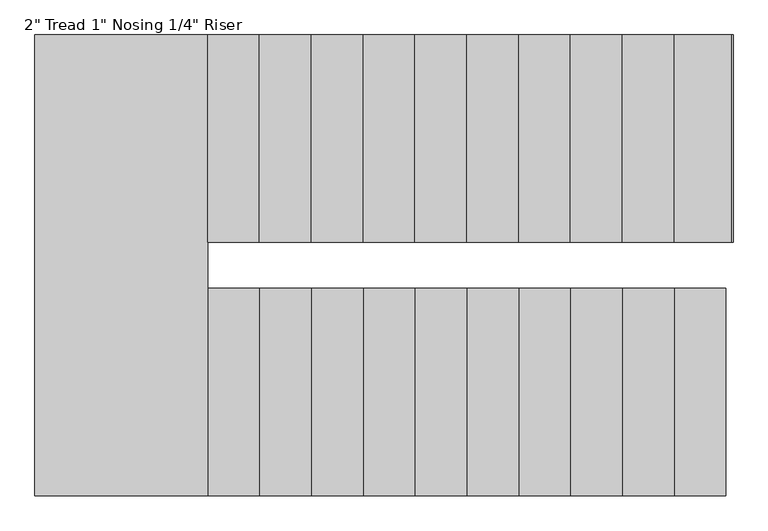
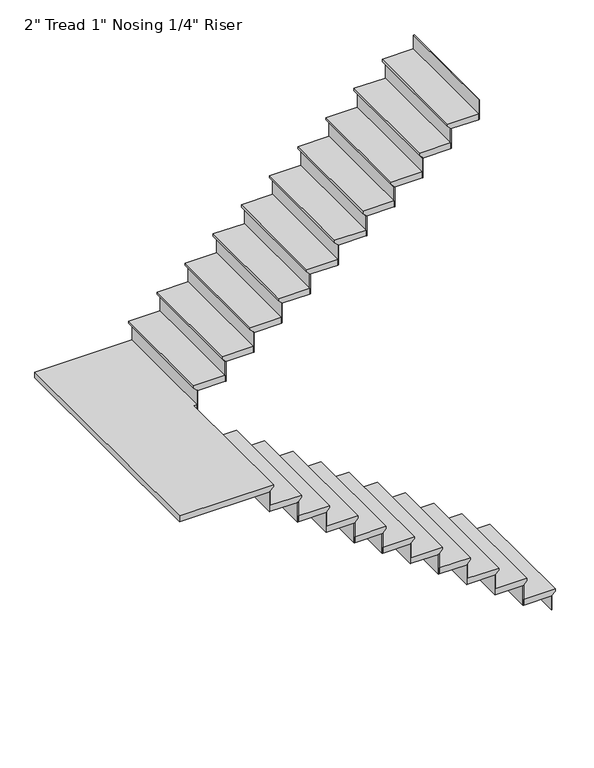
"""IFC4 building model written with IfcOpenShell, lengths in millimetres: stair flight geometry."""

from ifc_helpers import new_model, si_unit, origin, place, context, project, spatial, faceted_brep, source, transform, mapped, element, save


def stair_flight_66f938e6(model_context):
    return source(origin(), model_context, "Body", "Brep", [
        faceted_brep([(-2080.8410855, 332.1803617, 150.2833333), (-2080.8410855, 332.1803617, 169.3333333), (-2080.8410855, -582.2196383, 169.3333333), (-2080.8410855, -582.2196383, 150.2833333), (-2106.2410855, 332.1803617, 124.8833333), (-2106.2410855, -582.2196383, 124.8833333), (-2334.8410855, 332.1803617, 169.3333333), (-2334.8410855, -582.2196383, 169.3333333), (-2106.2410855, -582.2196383, 118.5333333), (-2334.8410855, -582.2196383, 118.5333333), (-2334.8410855, 332.1803617, 118.5333333), (-2106.2410855, 332.1803617, 118.5333333)], [[[0, 1, 2, 3]], [[4, 0, 3, 5]], [[2, 1, 6, 7]], [[8, 9, 10, 11]], [[2, 7, 9, 8, 5, 3]], [[8, 11, 4, 5]], [[6, 1, 0, 4, 11, 10]], [[7, 6, 10, 9]]]),
        faceted_brep([(-2106.2410855, 332.1803617, 118.5333333), (-2106.2410855, 332.1803617, 0.0), (-2112.5910855, 332.1803617, 0.0), (-2112.5910855, 332.1803617, 118.5333333), (-2106.2410855, -582.2196383, 118.5333333), (-2112.5910855, -582.2196383, 118.5333333), (-2112.5910855, -582.2196383, 0.0), (-2106.2410855, -582.2196383, 0.0)], [[[0, 1, 2, 3]], [[4, 5, 6, 7]], [[1, 0, 4, 7]], [[2, 1, 7, 6]], [[3, 2, 6, 5]], [[0, 3, 5, 4]]]),
        faceted_brep([(-2334.8410855, 332.1803617, 287.8666667), (-2334.8410855, 332.1803617, 118.5333333), (-2341.1910855, 332.1803617, 118.5333333), (-2341.1910855, 332.1803617, 287.8666667), (-2334.8410855, -582.2196383, 287.8666667), (-2341.1910855, -582.2196383, 287.8666667), (-2341.1910855, -582.2196383, 118.5333333), (-2334.8410855, -582.2196383, 118.5333333)], [[[0, 1, 2, 3]], [[4, 5, 6, 7]], [[1, 0, 4, 7]], [[2, 1, 7, 6]], [[3, 2, 6, 5]], [[0, 3, 5, 4]]]),
        faceted_brep([(-2309.4410855, -582.2196383, 338.6666667), (-2309.4410855, 332.1803617, 338.6666667), (-2563.4410855, 332.1803617, 338.6666667), (-2563.4410855, -582.2196383, 338.6666667), (-2334.8410855, -582.2196383, 287.8666667), (-2563.4410855, -582.2196383, 287.8666667), (-2563.4410855, 332.1803617, 287.8666667), (-2334.8410855, 332.1803617, 287.8666667), (-2334.8410855, -582.2196383, 294.2166667), (-2309.4410855, -582.2196383, 319.6166667), (-2334.8410855, 332.1803617, 294.2166667), (-2309.4410855, 332.1803617, 319.6166667)], [[[0, 1, 2, 3]], [[4, 5, 6, 7]], [[0, 3, 5, 4, 8, 9]], [[4, 7, 10, 8]], [[2, 1, 11, 10, 7, 6]], [[3, 2, 6, 5]], [[11, 1, 0, 9]], [[10, 11, 9, 8]]]),
        faceted_brep([(-2563.4410855, 332.1803617, 457.2), (-2563.4410855, 332.1803617, 287.8666667), (-2569.7910855, 332.1803617, 287.8666667), (-2569.7910855, 332.1803617, 457.2), (-2563.4410855, -582.2196383, 457.2), (-2569.7910855, -582.2196383, 457.2), (-2569.7910855, -582.2196383, 287.8666667), (-2563.4410855, -582.2196383, 287.8666667)], [[[0, 1, 2, 3]], [[4, 5, 6, 7]], [[1, 0, 4, 7]], [[2, 1, 7, 6]], [[3, 2, 6, 5]], [[0, 3, 5, 4]]]),
        faceted_brep([(-2538.0410855, -582.2196383, 508.0), (-2538.0410855, 332.1803617, 508.0), (-2792.0410855, 332.1803617, 508.0), (-2792.0410855, -582.2196383, 508.0), (-2563.4410855, -582.2196383, 457.2), (-2792.0410855, -582.2196383, 457.2), (-2792.0410855, 332.1803617, 457.2), (-2563.4410855, 332.1803617, 457.2), (-2563.4410855, -582.2196383, 463.55), (-2538.0410855, -582.2196383, 488.95), (-2563.4410855, 332.1803617, 463.55), (-2538.0410855, 332.1803617, 488.95)], [[[0, 1, 2, 3]], [[4, 5, 6, 7]], [[0, 3, 5, 4, 8, 9]], [[4, 7, 10, 8]], [[2, 1, 11, 10, 7, 6]], [[3, 2, 6, 5]], [[11, 1, 0, 9]], [[10, 11, 9, 8]]]),
        faceted_brep([(-2792.0410855, 332.1803617, 626.5333333), (-2792.0410855, 332.1803617, 457.2), (-2798.3910855, 332.1803617, 457.2), (-2798.3910855, 332.1803617, 626.5333333), (-2792.0410855, -582.2196383, 626.5333333), (-2798.3910855, -582.2196383, 626.5333333), (-2798.3910855, -582.2196383, 457.2), (-2792.0410855, -582.2196383, 457.2)], [[[0, 1, 2, 3]], [[4, 5, 6, 7]], [[1, 0, 4, 7]], [[2, 1, 7, 6]], [[3, 2, 6, 5]], [[0, 3, 5, 4]]]),
        faceted_brep([(-2766.6410855, -582.2196383, 677.3333333), (-2766.6410855, 332.1803617, 677.3333333), (-3020.6410855, 332.1803617, 677.3333333), (-3020.6410855, -582.2196383, 677.3333333), (-2792.0410855, -582.2196383, 626.5333333), (-3020.6410855, -582.2196383, 626.5333333), (-3020.6410855, 332.1803617, 626.5333333), (-2792.0410855, 332.1803617, 626.5333333), (-2792.0410855, -582.2196383, 632.8833333), (-2766.6410855, -582.2196383, 658.2833333), (-2792.0410855, 332.1803617, 632.8833333), (-2766.6410855, 332.1803617, 658.2833333)], [[[0, 1, 2, 3]], [[4, 5, 6, 7]], [[0, 3, 5, 4, 8, 9]], [[4, 7, 10, 8]], [[2, 1, 11, 10, 7, 6]], [[3, 2, 6, 5]], [[11, 1, 0, 9]], [[10, 11, 9, 8]]]),
        faceted_brep([(-3020.6410855, 332.1803617, 795.8666667), (-3020.6410855, 332.1803617, 626.5333333), (-3026.9910855, 332.1803617, 626.5333333), (-3026.9910855, 332.1803617, 795.8666667), (-3020.6410855, -582.2196383, 795.8666667), (-3026.9910855, -582.2196383, 795.8666667), (-3026.9910855, -582.2196383, 626.5333333), (-3020.6410855, -582.2196383, 626.5333333)], [[[0, 1, 2, 3]], [[4, 5, 6, 7]], [[1, 0, 4, 7]], [[2, 1, 7, 6]], [[3, 2, 6, 5]], [[0, 3, 5, 4]]]),
        faceted_brep([(-2995.2410855, -582.2196383, 846.6666667), (-2995.2410855, 332.1803617, 846.6666667), (-3249.2410855, 332.1803617, 846.6666667), (-3249.2410855, -582.2196383, 846.6666667), (-3020.6410855, -582.2196383, 795.8666667), (-3249.2410855, -582.2196383, 795.8666667), (-3249.2410855, 332.1803617, 795.8666667), (-3020.6410855, 332.1803617, 795.8666667), (-3020.6410855, -582.2196383, 802.2166667), (-2995.2410855, -582.2196383, 827.6166667), (-3020.6410855, 332.1803617, 802.2166667), (-2995.2410855, 332.1803617, 827.6166667)], [[[0, 1, 2, 3]], [[4, 5, 6, 7]], [[0, 3, 5, 4, 8, 9]], [[4, 7, 10, 8]], [[2, 1, 11, 10, 7, 6]], [[3, 2, 6, 5]], [[11, 1, 0, 9]], [[10, 11, 9, 8]]]),
        faceted_brep([(-3249.2410855, 332.1803617, 965.2), (-3249.2410855, 332.1803617, 795.8666667), (-3255.5910855, 332.1803617, 795.8666667), (-3255.5910855, 332.1803617, 965.2), (-3249.2410855, -582.2196383, 965.2), (-3255.5910855, -582.2196383, 965.2), (-3255.5910855, -582.2196383, 795.8666667), (-3249.2410855, -582.2196383, 795.8666667)], [[[0, 1, 2, 3]], [[4, 5, 6, 7]], [[1, 0, 4, 7]], [[2, 1, 7, 6]], [[3, 2, 6, 5]], [[0, 3, 5, 4]]]),
        faceted_brep([(-3223.8410855, -582.2196383, 1016.0), (-3223.8410855, 332.1803617, 1016.0), (-3477.8410855, 332.1803617, 1016.0), (-3477.8410855, -582.2196383, 1016.0), (-3249.2410855, -582.2196383, 965.2), (-3477.8410855, -582.2196383, 965.2), (-3477.8410855, 332.1803617, 965.2), (-3249.2410855, 332.1803617, 965.2), (-3249.2410855, -582.2196383, 971.55), (-3223.8410855, -582.2196383, 996.95), (-3249.2410855, 332.1803617, 971.55), (-3223.8410855, 332.1803617, 996.95)], [[[0, 1, 2, 3]], [[4, 5, 6, 7]], [[0, 3, 5, 4, 8, 9]], [[4, 7, 10, 8]], [[2, 1, 11, 10, 7, 6]], [[3, 2, 6, 5]], [[11, 1, 0, 9]], [[10, 11, 9, 8]]]),
        faceted_brep([(-3477.8410855, 332.1803617, 1134.5333333), (-3477.8410855, 332.1803617, 965.2), (-3484.1910855, 332.1803617, 965.2), (-3484.1910855, 332.1803617, 1134.5333333), (-3477.8410855, -582.2196383, 1134.5333333), (-3484.1910855, -582.2196383, 1134.5333333), (-3484.1910855, -582.2196383, 965.2), (-3477.8410855, -582.2196383, 965.2)], [[[0, 1, 2, 3]], [[4, 5, 6, 7]], [[1, 0, 4, 7]], [[2, 1, 7, 6]], [[3, 2, 6, 5]], [[0, 3, 5, 4]]]),
        faceted_brep([(-3452.4410855, -582.2196383, 1185.3333333), (-3452.4410855, 332.1803617, 1185.3333333), (-3706.4410855, 332.1803617, 1185.3333333), (-3706.4410855, -582.2196383, 1185.3333333), (-3477.8410855, -582.2196383, 1134.5333333), (-3706.4410855, -582.2196383, 1134.5333333), (-3706.4410855, 332.1803617, 1134.5333333), (-3477.8410855, 332.1803617, 1134.5333333), (-3477.8410855, -582.2196383, 1140.8833333), (-3452.4410855, -582.2196383, 1166.2833333), (-3477.8410855, 332.1803617, 1140.8833333), (-3452.4410855, 332.1803617, 1166.2833333)], [[[0, 1, 2, 3]], [[4, 5, 6, 7]], [[0, 3, 5, 4, 8, 9]], [[4, 7, 10, 8]], [[2, 1, 11, 10, 7, 6]], [[3, 2, 6, 5]], [[11, 1, 0, 9]], [[10, 11, 9, 8]]]),
        faceted_brep([(-3706.4410855, 332.1803617, 1303.8666667), (-3706.4410855, 332.1803617, 1134.5333333), (-3712.7910855, 332.1803617, 1134.5333333), (-3712.7910855, 332.1803617, 1303.8666667), (-3706.4410855, -582.2196383, 1303.8666667), (-3712.7910855, -582.2196383, 1303.8666667), (-3712.7910855, -582.2196383, 1134.5333333), (-3706.4410855, -582.2196383, 1134.5333333)], [[[0, 1, 2, 3]], [[4, 5, 6, 7]], [[1, 0, 4, 7]], [[2, 1, 7, 6]], [[3, 2, 6, 5]], [[0, 3, 5, 4]]]),
        faceted_brep([(-3681.0410855, -582.2196383, 1354.6666667), (-3681.0410855, 332.1803617, 1354.6666667), (-3935.0410855, 332.1803617, 1354.6666667), (-3935.0410855, -582.2196383, 1354.6666667), (-3706.4410855, -582.2196383, 1303.8666667), (-3935.0410855, -582.2196383, 1303.8666667), (-3935.0410855, 332.1803617, 1303.8666667), (-3706.4410855, 332.1803617, 1303.8666667), (-3706.4410855, -582.2196383, 1310.2166667), (-3681.0410855, -582.2196383, 1335.6166667), (-3706.4410855, 332.1803617, 1310.2166667), (-3681.0410855, 332.1803617, 1335.6166667)], [[[0, 1, 2, 3]], [[4, 5, 6, 7]], [[0, 3, 5, 4, 8, 9]], [[4, 7, 10, 8]], [[2, 1, 11, 10, 7, 6]], [[3, 2, 6, 5]], [[11, 1, 0, 9]], [[10, 11, 9, 8]]]),
        faceted_brep([(-3935.0410855, 332.1803617, 1473.2), (-3935.0410855, 332.1803617, 1303.8666667), (-3941.3910855, 332.1803617, 1303.8666667), (-3941.3910855, 332.1803617, 1473.2), (-3935.0410855, -582.2196383, 1473.2), (-3941.3910855, -582.2196383, 1473.2), (-3941.3910855, -582.2196383, 1303.8666667), (-3935.0410855, -582.2196383, 1303.8666667)], [[[0, 1, 2, 3]], [[4, 5, 6, 7]], [[1, 0, 4, 7]], [[2, 1, 7, 6]], [[3, 2, 6, 5]], [[0, 3, 5, 4]]]),
        faceted_brep([(-3909.6410855, -582.2196383, 1524.0), (-3909.6410855, 332.1803617, 1524.0), (-4163.6410855, 332.1803617, 1524.0), (-4163.6410855, -582.2196383, 1524.0), (-3935.0410855, -582.2196383, 1473.2), (-4163.6410855, -582.2196383, 1473.2), (-4163.6410855, 332.1803617, 1473.2), (-3935.0410855, 332.1803617, 1473.2), (-3935.0410855, -582.2196383, 1479.55), (-3909.6410855, -582.2196383, 1504.95), (-3935.0410855, 332.1803617, 1479.55), (-3909.6410855, 332.1803617, 1504.95)], [[[0, 1, 2, 3]], [[4, 5, 6, 7]], [[0, 3, 5, 4, 8, 9]], [[4, 7, 10, 8]], [[2, 1, 11, 10, 7, 6]], [[3, 2, 6, 5]], [[11, 1, 0, 9]], [[10, 11, 9, 8]]]),
        faceted_brep([(-4163.6410855, 332.1803617, 1642.5333333), (-4163.6410855, 332.1803617, 1473.2), (-4169.9910855, 332.1803617, 1473.2), (-4169.9910855, 332.1803617, 1642.5333333), (-4163.6410855, -582.2196383, 1642.5333333), (-4169.9910855, -582.2196383, 1642.5333333), (-4169.9910855, -582.2196383, 1473.2), (-4163.6410855, -582.2196383, 1473.2)], [[[0, 1, 2, 3]], [[4, 5, 6, 7]], [[1, 0, 4, 7]], [[2, 1, 7, 6]], [[3, 2, 6, 5]], [[0, 3, 5, 4]]]),
        faceted_brep([(-4138.2410855, -582.2196383, 1693.3333333), (-4138.2410855, 332.1803617, 1693.3333333), (-4392.2410855, 332.1803617, 1693.3333333), (-4392.2410855, -582.2196383, 1693.3333333), (-4163.6410855, -582.2196383, 1642.5333333), (-4392.2410855, -582.2196383, 1642.5333333), (-4392.2410855, 332.1803617, 1642.5333333), (-4163.6410855, 332.1803617, 1642.5333333), (-4163.6410855, -582.2196383, 1648.8833333), (-4138.2410855, -582.2196383, 1674.2833333), (-4163.6410855, 332.1803617, 1648.8833333), (-4138.2410855, 332.1803617, 1674.2833333)], [[[0, 1, 2, 3]], [[4, 5, 6, 7]], [[0, 3, 5, 4, 8, 9]], [[4, 7, 10, 8]], [[2, 1, 11, 10, 7, 6]], [[3, 2, 6, 5]], [[11, 1, 0, 9]], [[10, 11, 9, 8]]]),
        faceted_brep([(-4392.2410855, 332.1803617, 1811.8666667), (-4392.2410855, 332.1803617, 1642.5333333), (-4398.5910855, 332.1803617, 1642.5333333), (-4398.5910855, 332.1803617, 1811.8666667), (-4392.2410855, -582.2196383, 1811.8666667), (-4398.5910855, -582.2196383, 1811.8666667), (-4398.5910855, -582.2196383, 1642.5333333), (-4392.2410855, -582.2196383, 1642.5333333)], [[[0, 1, 2, 3]], [[4, 5, 6, 7]], [[1, 0, 4, 7]], [[2, 1, 7, 6]], [[3, 2, 6, 5]], [[0, 3, 5, 4]]]),
        faceted_brep([(-4341.4410855, 1449.7803617, 1862.6666667), (-5128.8410855, 1449.7803617, 1862.6666667), (-5128.8410855, -582.2196383, 1862.6666667), (-4366.8410855, -582.2196383, 1862.6666667), (-4366.8410855, 535.3803617, 1862.6666667), (-4341.4410855, 535.3803617, 1862.6666667), (-5128.8410855, 1449.7803617, 1811.8666667), (-4341.4410855, 1449.7803617, 1811.8666667), (-4341.4410855, 535.3803617, 1811.8666667), (-4366.8410855, 535.3803617, 1811.8666667), (-4366.8410855, 332.1803617, 1811.8666667), (-4392.2410855, 332.1803617, 1811.8666667), (-4392.2410855, -582.2196383, 1811.8666667), (-5128.8410855, -582.2196383, 1811.8666667), (-4392.2410855, -582.2196383, 1818.2166667), (-4366.8410855, -582.2196383, 1843.6166667), (-4392.2410855, 332.1803617, 1818.2166667), (-4366.8410855, 332.1803617, 1843.6166667)], [[[0, 1, 2, 3, 4, 5]], [[6, 7, 8, 9, 10, 11, 12, 13]], [[1, 0, 7, 6]], [[2, 1, 6, 13]], [[3, 2, 13, 12, 14, 15]], [[12, 11, 16, 14]], [[11, 10, 17, 16]], [[4, 3, 15, 17, 10, 9]], [[5, 4, 9, 8]], [[0, 5, 8, 7]], [[15, 14, 16, 17]]]),
        faceted_brep([(-4341.4410855, 535.3803617, 1981.2), (-4341.4410855, 535.3803617, 1811.8666667), (-4335.0910855, 535.3803617, 1811.8666667), (-4335.0910855, 535.3803617, 1981.2), (-4341.4410855, 1449.7803617, 1981.2), (-4335.0910855, 1449.7803617, 1981.2), (-4335.0910855, 1449.7803617, 1811.8666667), (-4341.4410855, 1449.7803617, 1811.8666667)], [[[0, 1, 2, 3]], [[4, 5, 6, 7]], [[1, 0, 4, 7]], [[2, 1, 7, 6]], [[3, 2, 6, 5]], [[0, 3, 5, 4]]]),
        faceted_brep([(-4366.8410855, 1449.7803617, 2032.0), (-4366.8410855, 535.3803617, 2032.0), (-4112.8410855, 535.3803617, 2032.0), (-4112.8410855, 1449.7803617, 2032.0), (-4341.4410855, 1449.7803617, 1981.2), (-4112.8410855, 1449.7803617, 1981.2), (-4112.8410855, 535.3803617, 1981.2), (-4341.4410855, 535.3803617, 1981.2), (-4341.4410855, 1449.7803617, 1987.55), (-4366.8410855, 1449.7803617, 2012.95), (-4341.4410855, 535.3803617, 1987.55), (-4366.8410855, 535.3803617, 2012.95)], [[[0, 1, 2, 3]], [[4, 5, 6, 7]], [[0, 3, 5, 4, 8, 9]], [[4, 7, 10, 8]], [[2, 1, 11, 10, 7, 6]], [[3, 2, 6, 5]], [[11, 1, 0, 9]], [[10, 11, 9, 8]]]),
        faceted_brep([(-4112.8410855, 535.3803617, 2150.5333333), (-4112.8410855, 535.3803617, 1981.2), (-4106.4910855, 535.3803617, 1981.2), (-4106.4910855, 535.3803617, 2150.5333333), (-4112.8410855, 1449.7803617, 2150.5333333), (-4106.4910855, 1449.7803617, 2150.5333333), (-4106.4910855, 1449.7803617, 1981.2), (-4112.8410855, 1449.7803617, 1981.2)], [[[0, 1, 2, 3]], [[4, 5, 6, 7]], [[1, 0, 4, 7]], [[2, 1, 7, 6]], [[3, 2, 6, 5]], [[0, 3, 5, 4]]]),
        faceted_brep([(-4138.2410855, 1449.7803617, 2201.3333333), (-4138.2410855, 535.3803617, 2201.3333333), (-3884.2410855, 535.3803617, 2201.3333333), (-3884.2410855, 1449.7803617, 2201.3333333), (-4112.8410855, 1449.7803617, 2150.5333333), (-3884.2410855, 1449.7803617, 2150.5333333), (-3884.2410855, 535.3803617, 2150.5333333), (-4112.8410855, 535.3803617, 2150.5333333), (-4112.8410855, 1449.7803617, 2156.8833333), (-4138.2410855, 1449.7803617, 2182.2833333), (-4112.8410855, 535.3803617, 2156.8833333), (-4138.2410855, 535.3803617, 2182.2833333)], [[[0, 1, 2, 3]], [[4, 5, 6, 7]], [[0, 3, 5, 4, 8, 9]], [[4, 7, 10, 8]], [[2, 1, 11, 10, 7, 6]], [[3, 2, 6, 5]], [[11, 1, 0, 9]], [[10, 11, 9, 8]]]),
        faceted_brep([(-3884.2410855, 535.3803617, 2319.8666667), (-3884.2410855, 535.3803617, 2150.5333333), (-3877.8910855, 535.3803617, 2150.5333333), (-3877.8910855, 535.3803617, 2319.8666667), (-3884.2410855, 1449.7803617, 2319.8666667), (-3877.8910855, 1449.7803617, 2319.8666667), (-3877.8910855, 1449.7803617, 2150.5333333), (-3884.2410855, 1449.7803617, 2150.5333333)], [[[0, 1, 2, 3]], [[4, 5, 6, 7]], [[1, 0, 4, 7]], [[2, 1, 7, 6]], [[3, 2, 6, 5]], [[0, 3, 5, 4]]]),
        faceted_brep([(-3909.6410855, 1449.7803617, 2370.6666667), (-3909.6410855, 535.3803617, 2370.6666667), (-3655.6410855, 535.3803617, 2370.6666667), (-3655.6410855, 1449.7803617, 2370.6666667), (-3884.2410855, 1449.7803617, 2319.8666667), (-3655.6410855, 1449.7803617, 2319.8666667), (-3655.6410855, 535.3803617, 2319.8666667), (-3884.2410855, 535.3803617, 2319.8666667), (-3884.2410855, 1449.7803617, 2326.2166667), (-3909.6410855, 1449.7803617, 2351.6166667), (-3884.2410855, 535.3803617, 2326.2166667), (-3909.6410855, 535.3803617, 2351.6166667)], [[[0, 1, 2, 3]], [[4, 5, 6, 7]], [[0, 3, 5, 4, 8, 9]], [[4, 7, 10, 8]], [[2, 1, 11, 10, 7, 6]], [[3, 2, 6, 5]], [[11, 1, 0, 9]], [[10, 11, 9, 8]]]),
        faceted_brep([(-3655.6410855, 535.3803617, 2489.2), (-3655.6410855, 535.3803617, 2319.8666667), (-3649.2910855, 535.3803617, 2319.8666667), (-3649.2910855, 535.3803617, 2489.2), (-3655.6410855, 1449.7803617, 2489.2), (-3649.2910855, 1449.7803617, 2489.2), (-3649.2910855, 1449.7803617, 2319.8666667), (-3655.6410855, 1449.7803617, 2319.8666667)], [[[0, 1, 2, 3]], [[4, 5, 6, 7]], [[1, 0, 4, 7]], [[2, 1, 7, 6]], [[3, 2, 6, 5]], [[0, 3, 5, 4]]]),
        faceted_brep([(-3681.0410855, 1449.7803617, 2540.0), (-3681.0410855, 535.3803617, 2540.0), (-3427.0410855, 535.3803617, 2540.0), (-3427.0410855, 1449.7803617, 2540.0), (-3655.6410855, 1449.7803617, 2489.2), (-3427.0410855, 1449.7803617, 2489.2), (-3427.0410855, 535.3803617, 2489.2), (-3655.6410855, 535.3803617, 2489.2), (-3655.6410855, 1449.7803617, 2495.55), (-3681.0410855, 1449.7803617, 2520.95), (-3655.6410855, 535.3803617, 2495.55), (-3681.0410855, 535.3803617, 2520.95)], [[[0, 1, 2, 3]], [[4, 5, 6, 7]], [[0, 3, 5, 4, 8, 9]], [[4, 7, 10, 8]], [[2, 1, 11, 10, 7, 6]], [[3, 2, 6, 5]], [[11, 1, 0, 9]], [[10, 11, 9, 8]]]),
        faceted_brep([(-3427.0410855, 535.3803617, 2658.5333333), (-3427.0410855, 535.3803617, 2489.2), (-3420.6910855, 535.3803617, 2489.2), (-3420.6910855, 535.3803617, 2658.5333333), (-3427.0410855, 1449.7803617, 2658.5333333), (-3420.6910855, 1449.7803617, 2658.5333333), (-3420.6910855, 1449.7803617, 2489.2), (-3427.0410855, 1449.7803617, 2489.2)], [[[0, 1, 2, 3]], [[4, 5, 6, 7]], [[1, 0, 4, 7]], [[2, 1, 7, 6]], [[3, 2, 6, 5]], [[0, 3, 5, 4]]]),
        faceted_brep([(-3452.4410855, 1449.7803617, 2709.3333333), (-3452.4410855, 535.3803617, 2709.3333333), (-3198.4410855, 535.3803617, 2709.3333333), (-3198.4410855, 1449.7803617, 2709.3333333), (-3427.0410855, 1449.7803617, 2658.5333333), (-3198.4410855, 1449.7803617, 2658.5333333), (-3198.4410855, 535.3803617, 2658.5333333), (-3427.0410855, 535.3803617, 2658.5333333), (-3427.0410855, 1449.7803617, 2664.8833333), (-3452.4410855, 1449.7803617, 2690.2833333), (-3427.0410855, 535.3803617, 2664.8833333), (-3452.4410855, 535.3803617, 2690.2833333)], [[[0, 1, 2, 3]], [[4, 5, 6, 7]], [[0, 3, 5, 4, 8, 9]], [[4, 7, 10, 8]], [[2, 1, 11, 10, 7, 6]], [[3, 2, 6, 5]], [[11, 1, 0, 9]], [[10, 11, 9, 8]]]),
        faceted_brep([(-3198.4410855, 535.3803617, 2827.8666667), (-3198.4410855, 535.3803617, 2658.5333333), (-3192.0910855, 535.3803617, 2658.5333333), (-3192.0910855, 535.3803617, 2827.8666667), (-3198.4410855, 1449.7803617, 2827.8666667), (-3192.0910855, 1449.7803617, 2827.8666667), (-3192.0910855, 1449.7803617, 2658.5333333), (-3198.4410855, 1449.7803617, 2658.5333333)], [[[0, 1, 2, 3]], [[4, 5, 6, 7]], [[1, 0, 4, 7]], [[2, 1, 7, 6]], [[3, 2, 6, 5]], [[0, 3, 5, 4]]]),
        faceted_brep([(-3223.8410855, 1449.7803617, 2878.6666667), (-3223.8410855, 535.3803617, 2878.6666667), (-2969.8410855, 535.3803617, 2878.6666667), (-2969.8410855, 1449.7803617, 2878.6666667), (-3198.4410855, 1449.7803617, 2827.8666667), (-2969.8410855, 1449.7803617, 2827.8666667), (-2969.8410855, 535.3803617, 2827.8666667), (-3198.4410855, 535.3803617, 2827.8666667), (-3198.4410855, 1449.7803617, 2834.2166667), (-3223.8410855, 1449.7803617, 2859.6166667), (-3198.4410855, 535.3803617, 2834.2166667), (-3223.8410855, 535.3803617, 2859.6166667)], [[[0, 1, 2, 3]], [[4, 5, 6, 7]], [[0, 3, 5, 4, 8, 9]], [[4, 7, 10, 8]], [[2, 1, 11, 10, 7, 6]], [[3, 2, 6, 5]], [[11, 1, 0, 9]], [[10, 11, 9, 8]]]),
        faceted_brep([(-2969.8410855, 535.3803617, 2997.2), (-2969.8410855, 535.3803617, 2827.8666667), (-2963.4910855, 535.3803617, 2827.8666667), (-2963.4910855, 535.3803617, 2997.2), (-2969.8410855, 1449.7803617, 2997.2), (-2963.4910855, 1449.7803617, 2997.2), (-2963.4910855, 1449.7803617, 2827.8666667), (-2969.8410855, 1449.7803617, 2827.8666667)], [[[0, 1, 2, 3]], [[4, 5, 6, 7]], [[1, 0, 4, 7]], [[2, 1, 7, 6]], [[3, 2, 6, 5]], [[0, 3, 5, 4]]]),
        faceted_brep([(-2995.2410855, 1449.7803617, 3048.0), (-2995.2410855, 535.3803617, 3048.0), (-2741.2410855, 535.3803617, 3048.0), (-2741.2410855, 1449.7803617, 3048.0), (-2969.8410855, 1449.7803617, 2997.2), (-2741.2410855, 1449.7803617, 2997.2), (-2741.2410855, 535.3803617, 2997.2), (-2969.8410855, 535.3803617, 2997.2), (-2969.8410855, 1449.7803617, 3003.55), (-2995.2410855, 1449.7803617, 3028.95), (-2969.8410855, 535.3803617, 3003.55), (-2995.2410855, 535.3803617, 3028.95)], [[[0, 1, 2, 3]], [[4, 5, 6, 7]], [[0, 3, 5, 4, 8, 9]], [[4, 7, 10, 8]], [[2, 1, 11, 10, 7, 6]], [[3, 2, 6, 5]], [[11, 1, 0, 9]], [[10, 11, 9, 8]]]),
        faceted_brep([(-2741.2410855, 535.3803617, 3166.5333333), (-2741.2410855, 535.3803617, 2997.2), (-2734.8910855, 535.3803617, 2997.2), (-2734.8910855, 535.3803617, 3166.5333333), (-2741.2410855, 1449.7803617, 3166.5333333), (-2734.8910855, 1449.7803617, 3166.5333333), (-2734.8910855, 1449.7803617, 2997.2), (-2741.2410855, 1449.7803617, 2997.2)], [[[0, 1, 2, 3]], [[4, 5, 6, 7]], [[1, 0, 4, 7]], [[2, 1, 7, 6]], [[3, 2, 6, 5]], [[0, 3, 5, 4]]]),
        faceted_brep([(-2766.6410855, 1449.7803617, 3217.3333333), (-2766.6410855, 535.3803617, 3217.3333333), (-2512.6410855, 535.3803617, 3217.3333333), (-2512.6410855, 1449.7803617, 3217.3333333), (-2741.2410855, 1449.7803617, 3166.5333333), (-2512.6410855, 1449.7803617, 3166.5333333), (-2512.6410855, 535.3803617, 3166.5333333), (-2741.2410855, 535.3803617, 3166.5333333), (-2741.2410855, 1449.7803617, 3172.8833333), (-2766.6410855, 1449.7803617, 3198.2833333), (-2741.2410855, 535.3803617, 3172.8833333), (-2766.6410855, 535.3803617, 3198.2833333)], [[[0, 1, 2, 3]], [[4, 5, 6, 7]], [[0, 3, 5, 4, 8, 9]], [[4, 7, 10, 8]], [[2, 1, 11, 10, 7, 6]], [[3, 2, 6, 5]], [[11, 1, 0, 9]], [[10, 11, 9, 8]]]),
        faceted_brep([(-2512.6410855, 535.3803617, 3335.8666667), (-2512.6410855, 535.3803617, 3166.5333333), (-2506.2910855, 535.3803617, 3166.5333333), (-2506.2910855, 535.3803617, 3335.8666667), (-2512.6410855, 1449.7803617, 3335.8666667), (-2506.2910855, 1449.7803617, 3335.8666667), (-2506.2910855, 1449.7803617, 3166.5333333), (-2512.6410855, 1449.7803617, 3166.5333333)], [[[0, 1, 2, 3]], [[4, 5, 6, 7]], [[1, 0, 4, 7]], [[2, 1, 7, 6]], [[3, 2, 6, 5]], [[0, 3, 5, 4]]]),
        faceted_brep([(-2538.0410855, 1449.7803617, 3386.6666667), (-2538.0410855, 535.3803617, 3386.6666667), (-2284.0410855, 535.3803617, 3386.6666667), (-2284.0410855, 1449.7803617, 3386.6666667), (-2512.6410855, 1449.7803617, 3335.8666667), (-2284.0410855, 1449.7803617, 3335.8666667), (-2284.0410855, 535.3803617, 3335.8666667), (-2512.6410855, 535.3803617, 3335.8666667), (-2512.6410855, 1449.7803617, 3342.2166667), (-2538.0410855, 1449.7803617, 3367.6166667), (-2512.6410855, 535.3803617, 3342.2166667), (-2538.0410855, 535.3803617, 3367.6166667)], [[[0, 1, 2, 3]], [[4, 5, 6, 7]], [[0, 3, 5, 4, 8, 9]], [[4, 7, 10, 8]], [[2, 1, 11, 10, 7, 6]], [[3, 2, 6, 5]], [[11, 1, 0, 9]], [[10, 11, 9, 8]]]),
        faceted_brep([(-2284.0410855, 535.3803617, 3505.2), (-2284.0410855, 535.3803617, 3335.8666667), (-2277.6910855, 535.3803617, 3335.8666667), (-2277.6910855, 535.3803617, 3505.2), (-2284.0410855, 1449.7803617, 3505.2), (-2277.6910855, 1449.7803617, 3505.2), (-2277.6910855, 1449.7803617, 3335.8666667), (-2284.0410855, 1449.7803617, 3335.8666667)], [[[0, 1, 2, 3]], [[4, 5, 6, 7]], [[1, 0, 4, 7]], [[2, 1, 7, 6]], [[3, 2, 6, 5]], [[0, 3, 5, 4]]]),
        faceted_brep([(-2055.4410855, 535.3803617, 3674.5333333), (-2055.4410855, 535.3803617, 3505.2), (-2049.0910855, 535.3803617, 3505.2), (-2049.0910855, 535.3803617, 3674.5333333), (-2055.4410855, 1449.7803617, 3674.5333333), (-2049.0910855, 1449.7803617, 3674.5333333), (-2049.0910855, 1449.7803617, 3505.2), (-2055.4410855, 1449.7803617, 3505.2)], [[[0, 1, 2, 3]], [[4, 5, 6, 7]], [[1, 0, 4, 7]], [[2, 1, 7, 6]], [[3, 2, 6, 5]], [[0, 3, 5, 4]]]),
        faceted_brep([(-2309.4410855, 1449.7803617, 3556.0), (-2309.4410855, 535.3803617, 3556.0), (-2055.4410855, 535.3803617, 3556.0), (-2055.4410855, 1449.7803617, 3556.0), (-2284.0410855, 1449.7803617, 3505.2), (-2055.4410855, 1449.7803617, 3505.2), (-2055.4410855, 535.3803617, 3505.2), (-2284.0410855, 535.3803617, 3505.2), (-2284.0410855, 1449.7803617, 3511.55), (-2309.4410855, 1449.7803617, 3536.95), (-2284.0410855, 535.3803617, 3511.55), (-2309.4410855, 535.3803617, 3536.95)], [[[0, 1, 2, 3]], [[4, 5, 6, 7]], [[0, 3, 5, 4, 8, 9]], [[4, 7, 10, 8]], [[2, 1, 11, 10, 7, 6]], [[3, 2, 6, 5]], [[11, 1, 0, 9]], [[10, 11, 9, 8]]]),
    ])


if __name__ == "__main__":
    model = new_model("IFC4")
    model_context = context("Model", 3, world=origin())
    ifc_project = project(units=[si_unit("LENGTHUNIT", "METRE", prefix="MILLI")], contexts=[model_context])
    site = spatial("IfcSite", under=ifc_project)
    building = spatial("IfcBuilding", under=site)
    placement = place(None, origin())
    stair_flight_shape = stair_flight_66f938e6(model_context)
    element("IfcStairFlight", 1, ObjectType="2\" Tread 1\" Nosing 1/4\" Riser", at=placement, inside=building, context=model_context, shape_type="MappedRepresentation", body=[
        mapped(stair_flight_shape, transform((0.0, 0.0, 0.0), x_axis=(1.0, 0.0, 0.0), y_axis=(0.0, 1.0, 0.0), z_axis=(0.0, 0.0, 1.0))),
    ])
    save(model, "model.ifc")
